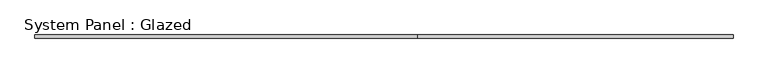
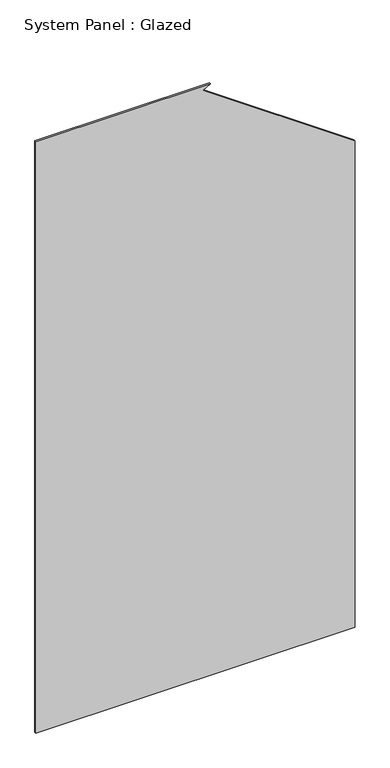
"""IFC4 building model written with IfcOpenShell, lengths in millimetres: plate geometry, System Panel : Glazed."""

from ifc_helpers import new_model, si_unit, frame, origin, place, context, project, spatial, polyline, outline, extrude, source, transform, mapped, element, save


def system_panel_glazed_5205d833(model_context):
    return source(origin(), model_context, "Body", "SweptSolid", [
        extrude(outline(polyline([(0.0, -600.0), (0.0, 600.0), (1934.0339089, 600.0), (2334.0423978, 28.728674), (2350.0, 57.4074958), (2350.0, -600.0), (0.0, -600.0)])), frame((0.0, 34.0, 0.0), z_axis=(0.0, 1.0, 0.0), x_axis=(0.0, 0.0, 1.0)), (0.0, 0.0, 1.0), 6.0),
    ])


if __name__ == "__main__":
    model = new_model("IFC4")
    model_context = context("Model", 3, world=origin())
    ifc_project = project(units=[si_unit("LENGTHUNIT", "METRE", prefix="MILLI")], contexts=[model_context])
    site = spatial("IfcSite", under=ifc_project)
    building = spatial("IfcBuilding", under=site)
    placement = place(None, origin())
    system_panel_glazed_shape = system_panel_glazed_5205d833(model_context)
    element("IfcPlate", 1, ObjectType="System Panel : Glazed", at=placement, inside=building, context=model_context, shape_type="MappedRepresentation", body=[
        mapped(system_panel_glazed_shape, transform((0.0, 0.0, 0.0), x_axis=(1.0, 0.0, 0.0), y_axis=(0.0, 1.0, 0.0), z_axis=(0.0, 0.0, 1.0))),
    ])
    save(model, "model.ifc")

# Revit data of these elements
# Type "System Panel : Glazed"
#   Construction Type Id = "GSP4R"
#   Analytic Construction = "1/8 in Pilkington single glazing"
#   Visual Light Transmittance = 0.9
#   Solar Heat Gain Coefficient = 0.86
#   Heat Transfer Coefficient (U) = 6.7069 W/(m²·K)
#   Define Thermal Properties by = 1
# Element 1 (IfcPlate, "System Panel : Glazed")
#   Materials on its faces: "Default New Material(6)"
# Materials
#   "Default New Material(6)": class "Generic", colour RGB 191 25 25, transparency 0.9, Cost = 0
